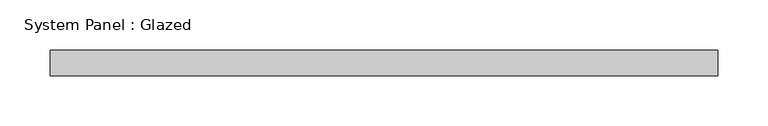
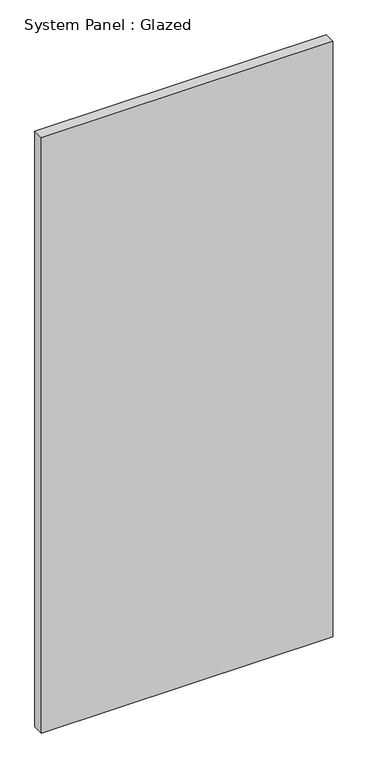
"""IFC4 building model written with IfcOpenShell, lengths in millimetres: plate geometry, System Panel : Glazed."""

from ifc_helpers import new_model, si_unit, origin, origin_with_axes, place, context, project, spatial, polyline, outline, extrude, source, transform, mapped, element, save


def system_panel_glazed_de152a88(model_context):
    return source(origin(), model_context, "Body", "SweptSolid", [
        extrude(outline(polyline([(333.375, 19.05), (-333.375, 19.05), (-333.375, 44.45), (333.375, 44.45), (333.375, 19.05)])), origin_with_axes(), (0.0, 0.0, 1.0), 1439.9800364),
    ])


if __name__ == "__main__":
    model = new_model("IFC4")
    model_context = context("Model", 3, world=origin())
    ifc_project = project(units=[si_unit("LENGTHUNIT", "METRE", prefix="MILLI")], contexts=[model_context])
    site = spatial("IfcSite", under=ifc_project)
    building = spatial("IfcBuilding", under=site)
    placement = place(None, origin())
    system_panel_glazed_shape = system_panel_glazed_de152a88(model_context)
    element("IfcPlate", 1, ObjectType="System Panel : Glazed", at=placement, inside=building, context=model_context, shape_type="MappedRepresentation", body=[
        mapped(system_panel_glazed_shape, transform((0.0, 0.0, 0.0), x_axis=(1.0, 0.0, 0.0), y_axis=(0.0, 1.0, 0.0), z_axis=(0.0, 0.0, 1.0))),
    ])
    save(model, "model.ifc")

# Revit data of these elements
# Type "System Panel : Glazed"
#   Construction Type Id = "GSP4R"
#   Analytic Construction = "1/8 in Pilkington single glazing"
#   Visual Light Transmittance = 0.9
#   Solar Heat Gain Coefficient = 0.86
#   Heat Transfer Coefficient (U) = 1.18115 BTU/(h·ft²·°F)
#   Define Thermal Properties by = 1
# Element 1 (IfcPlate, "System Panel : Glazed")
#   Materials on its faces: "Glass"
# Materials
#   "Glass": class "Glass", colour RGB 0 128 192, transparency 0.75, Description = "Soda Lime Glass", Cost = 0
